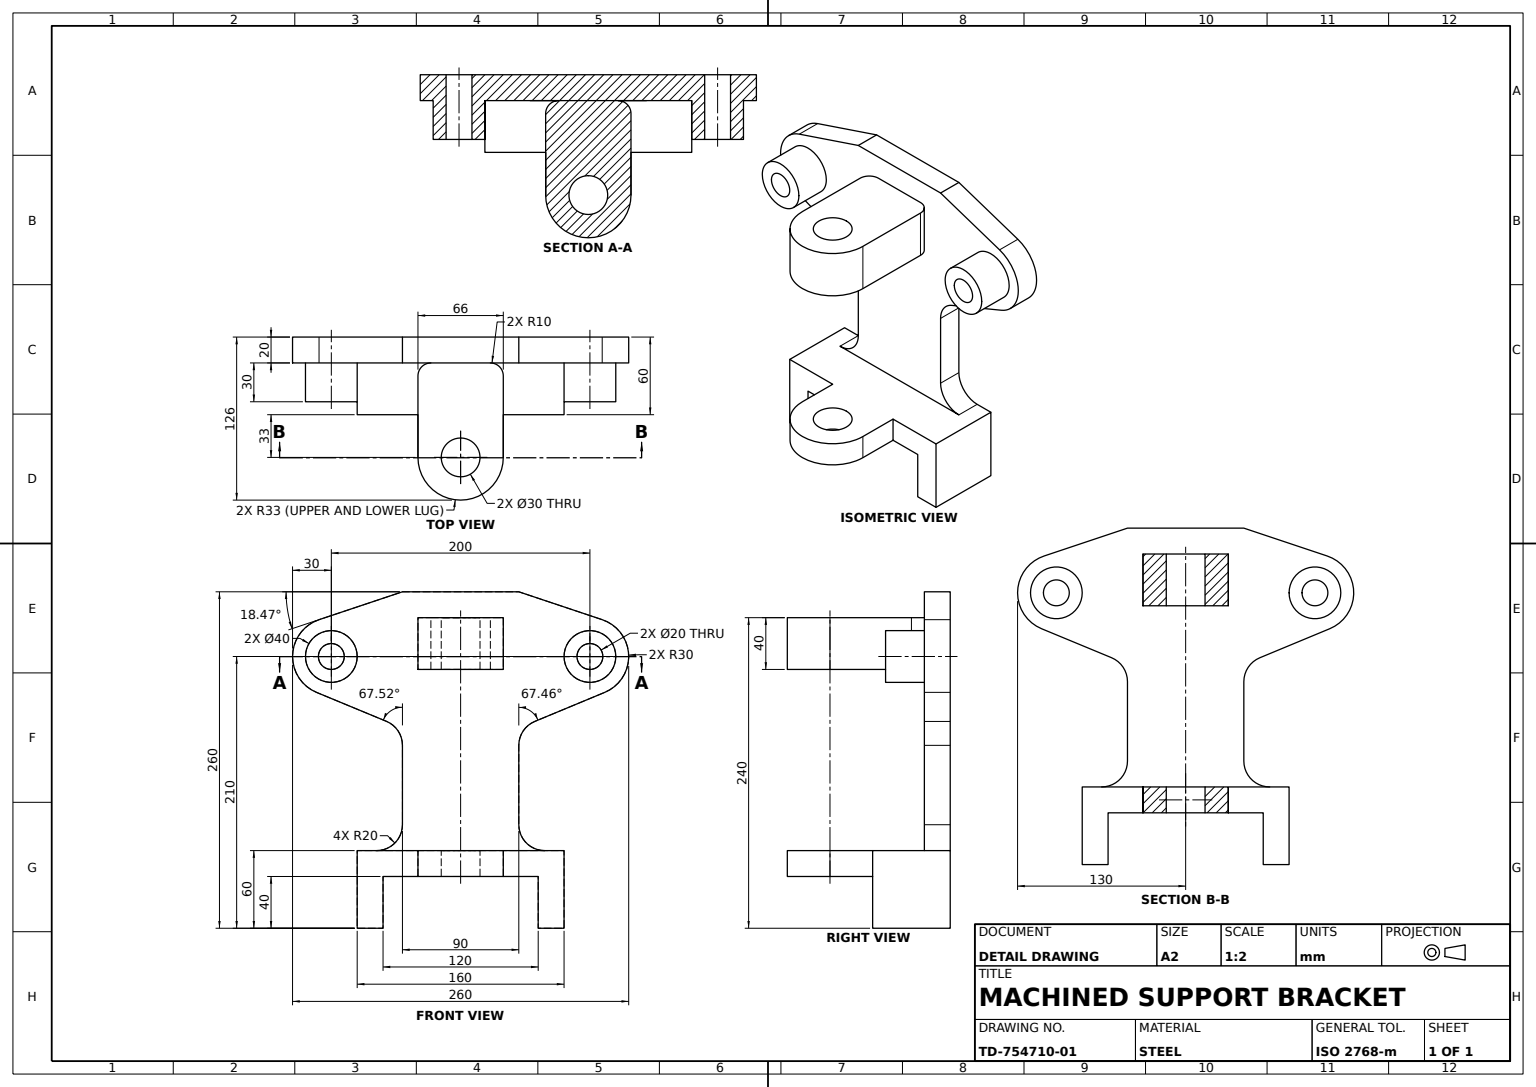
from build123d import *

# Parameters (mm, degrees)
BASE_WEB_DEPTH             = 60
UPPER_LUG_DEPTH            = 20
UPPER_LUG_BORE_SKETCH_R    = 15
UPPER_LUG_BORE_30_DEPTH    = 20
MOUNTING_FLANGE_DEPTH      = 20
FLANGE_BOSSES_SKETCH_R     = 20
FLANGE_BOSSES_SKETCH_R_2   = 10
FLANGE_BOSSES_DEPTH        = 30
LOWER_LUG_SKETCH_R         = 15
LOWER_LUG_DEPTH            = 40
FLANGE_START               = -40
FLANGE_BOSS_HOLES_SKETCH_R = 10
FLANGE_BOSS_HOLES_DEPTH    = 40


with BuildPart() as part:
    # Base Web Sketch → Base Web (new body)
    with BuildSketch(Plane.XY):
        Polygon((0, 0), (0, 60), (160, 60), (160, 0), (140, 0), (140, 40), (20, 40), (20, 0), align=None)
    extrude(amount=BASE_WEB_DEPTH)

    # Upper Lug Sketch → Upper Lug (add)
    with BuildSketch(Plane(origin=(0, 60, 0), x_dir=(1, 0, 0), z_dir=(0, 1, 0))):
        with BuildLine():
            Line((47, -93), (47, -60))
            Line((47, -60), (113, -60))
            Line((113, -60), (113, -93))
            ThreePointArc((113, -93), (80, -126), (47, -93))
        make_face()
    extrude(amount=-UPPER_LUG_DEPTH)

    # Upper Lug Bore Sketch → Upper Lug Bore Ø30 (cut)
    with BuildSketch(Plane(origin=(0, 60, 0), x_dir=(1, 0, 0), z_dir=(0, 1, 0))):
        with Locations(Location((80, -93, 0), (0, 0, 270))):
            Circle(UPPER_LUG_BORE_SKETCH_R)
    extrude(amount=-UPPER_LUG_BORE_30_DEPTH, mode=Mode.SUBTRACT)

    # Mounting Flange Sketch → Mounting Flange (add)
    with BuildSketch(Plane.XY):
        with BuildLine():
            Line((15, 60), (145, 60))
            ThreePointArc((145, 60), (130.857864376, 65.857864376), (125, 80))
            Line((125, 80), (125, 141.339700933))
            ThreePointArc((125, 141.339700933), (128.366825359, 152.445442752), (137.333750135, 159.812075252))
            Line((137.333750135, 159.812075252), (191.499374797, 182.29143852))
            ThreePointArc((191.499374797, 182.29143852), (209.981089089, 211.065033817), (189.504258609, 238.45468447))
            Line((189.504258609, 238.45468447), (125, 260))
            Line((125, 260), (35, 260))
            Line((35, 260), (-29.504258609, 238.45468447))
            ThreePointArc((-29.504258609, 238.45468447), (-49.981644615, 211.049278887), (-31.470247269, 182.279368197))
            Line((-31.470247269, 182.279368197), (22.646831513, 159.886795057))
            ThreePointArc((22.646831513, 159.886795057), (31.627336381, 152.520854718), (35, 141.406373855))
            Line((35, 141.406373855), (35, 80))
            ThreePointArc((35, 80), (29.142135624, 65.857864376), (15, 60))
        make_face()
    extrude(amount=MOUNTING_FLANGE_DEPTH)

    # Flange Bosses Sketch → Flange Bosses (add)
    # profile 1 of 2: a face of its own
    with BuildSketch(Plane.XY.offset(20)):
        with Locations((-20, 210)):
            Circle(FLANGE_BOSSES_SKETCH_R)
        with Locations((-20, 210)):
            Circle(FLANGE_BOSSES_SKETCH_R_2, mode=Mode.SUBTRACT)
    # profile 2 of 2: a face of its own
    with BuildSketch(Plane.XY.offset(20)):
        with Locations((180, 210)):
            Circle(FLANGE_BOSSES_SKETCH_R)
        with Locations((180, 210)):
            Circle(FLANGE_BOSSES_SKETCH_R_2, mode=Mode.SUBTRACT)
    extrude(amount=FLANGE_BOSSES_DEPTH)

    # Lower Lug Sketch → Lower Lug (add)
    with BuildSketch(Plane(origin=(0, 240, 0), x_dir=(1, 0, 0), z_dir=(0, 1, 0))):
        with BuildLine():
            Line((47, -93), (47, -30))
            ThreePointArc((47, -30), (49.928932188, -22.928932188), (57, -20))
            Line((57, -20), (103, -20))
            ThreePointArc((103, -20), (110.071067812, -22.928932188), (113, -30))
            Line((113, -30), (113, -93))
            ThreePointArc((113, -93), (80, -126), (47, -93))
        make_face()
        with Locations(Location((80, -93, 0), (0, 0, 270))):
            Circle(LOWER_LUG_SKETCH_R, mode=Mode.SUBTRACT)
    extrude(amount=-LOWER_LUG_DEPTH)

    # Flange Boss Holes Sketch → Flange Boss Holes (cut)
    with BuildSketch(Plane.XY.offset(20).offset(FLANGE_START)):
        with Locations(Location((-20, 210, 0), (0, 0, 180))):
            Circle(FLANGE_BOSS_HOLES_SKETCH_R)
        with Locations(Location((180, 210, 0), (0, 0, 180))):
            Circle(FLANGE_BOSS_HOLES_SKETCH_R)
    extrude(amount=FLANGE_BOSS_HOLES_DEPTH, mode=Mode.SUBTRACT)


solid = part.part
